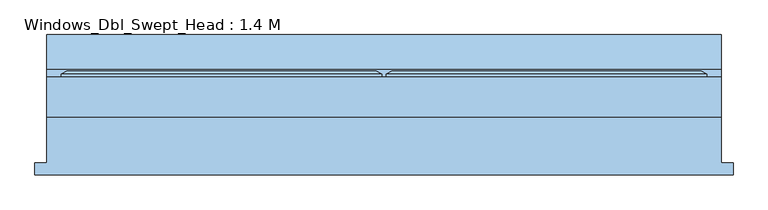
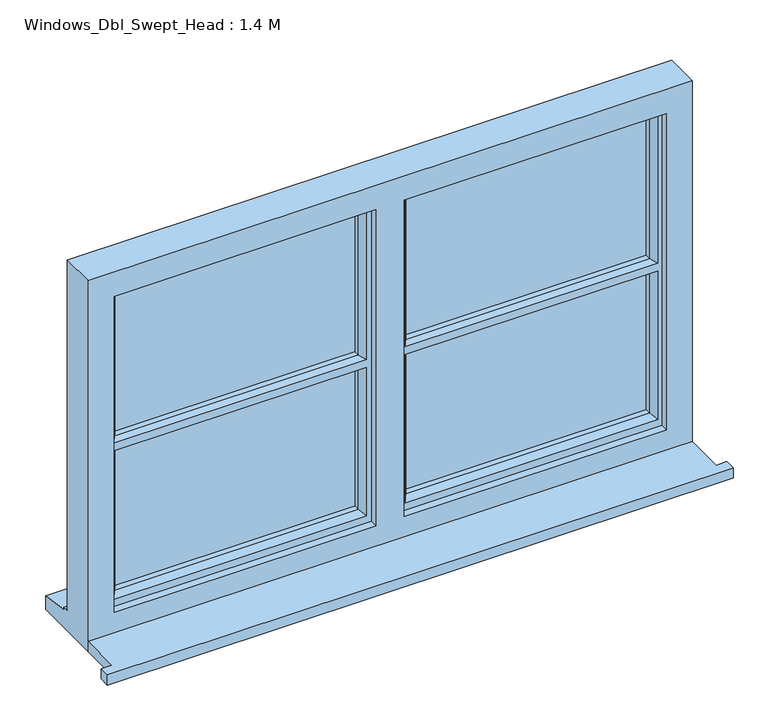
"""IFC4 building model written with IfcOpenShell, lengths in millimetres: window geometry, Windows_Dbl_Swept_Head : 1.4 M."""

from ifc_helpers import new_model, si_unit, frame, origin, place, context, project, spatial, polyline, circle_curve, outline, extrude, faceted_brep, source, transform, mapped, element, save
from ifc_brep_helpers import plane_surface, revolved_surface, advanced_brep


def windows_dbl_swept_head_1_4_m_8667dff2(model_context):
    return source(origin(), model_context, "Body", "SolidModel", [
        extrude(outline(polyline([(-1010.0, -130.8434322), (-1010.0, -105.8434322), (-985.0, -105.8434322), (-985.0, -10.2434322), (415.0, -10.2434322), (415.0, -105.8434322), (440.0, -105.8434322), (440.0, -130.8434322), (-1010.0, -130.8434322)])), frame((0.0, 0.0, 1200.0), z_axis=(0.0, 0.0, 1.0), x_axis=(1.0, 0.0, 0.0)), (0.0, 0.0, 1.0), 25.0),
        extrude(outline(polyline([(345.1480377, 36.7565678), (-240.0, 36.7565678), (-240.0, 60.7565678), (345.1480377, 60.7565678), (345.1480377, 36.7565678)])), frame((0.0, 0.0, 1293.0), z_axis=(0.0, 0.0, 1.0), x_axis=(1.0, 0.0, 0.0)), (0.0, 0.0, 1.0), 365.5),
        extrude(outline(polyline([(345.1480377, 36.7565678), (-240.0, 36.7565678), (-240.0, 60.7565678), (345.1480377, 60.7565678), (345.1480377, 36.7565678)])), frame((0.0, 0.0, 1674.5), z_axis=(0.0, 0.0, 1.0), x_axis=(1.0, 0.0, 0.0)), (0.0, 0.0, 1.0), 365.5),
        extrude(outline(polyline([(-330.0, 36.7565678), (-915.0, 36.7565678), (-915.0, 60.7565678), (-330.0, 60.7565678), (-330.0, 36.7565678)])), frame((0.0, 0.0, 1674.5), z_axis=(0.0, 0.0, 1.0), x_axis=(1.0, 0.0, 0.0)), (0.0, 0.0, 1.0), 365.5),
        extrude(outline(polyline([(-330.0, 36.7565678), (-915.1480377, 36.7565678), (-915.1480377, 60.7565678), (-330.0, 60.7565678), (-330.0, 36.7565678)])), frame((0.0, 0.0, 1292.8519623), z_axis=(0.0, 0.0, 1.0), x_axis=(1.0, 0.0, 0.0)), (0.0, 0.0, 1.0), 365.6480377),
        faceted_brep([(-985.0, -10.2434322, 1200.0), (415.0, -10.2434322, 1200.0), (415.0, -10.2434322, 2110.0), (-985.0, -10.2434322, 2110.0), (-318.0, -10.2434322, 2050.0), (-318.0, -10.2434322, 1275.0), (-925.0, -10.2434322, 1275.0), (-925.0, -10.2434322, 2050.0), (-252.0, -10.2434322, 2050.0), (355.0, -10.2434322, 2050.0), (355.0, -10.2434322, 1275.0), (-252.0, -10.2434322, 1275.0), (-985.0, 72.7565678, 2110.0), (-985.0, 72.7565678, 1251.0), (-985.0, 87.7565678, 1249.68767), (-985.0, 87.7565678, 1244.7449676), (-985.0, 160.2565678, 1233.8088847), (-985.0, 160.2565678, 1200.0), (415.0, 72.7565678, 2110.0), (415.0, 72.7565678, 1251.0), (-945.0, 72.7565678, 2070.0), (-945.0, 72.7565678, 1263.0), (-300.0, 72.7565678, 1263.0), (-300.0, 72.7565678, 2070.0), (-270.0, 72.7565678, 2070.0), (-270.0, 72.7565678, 1263.0), (375.0, 72.7565678, 1263.0), (375.0, 72.7565678, 2070.0), (-945.0, 7.7565678, 2070.0), (-945.0, 7.7565678, 1263.0), (-300.0, 7.7565678, 2070.0), (-300.0, 7.7565678, 1263.0), (-318.0, 7.7565678, 2050.0), (-925.0, 7.7565678, 2050.0), (-925.0, 7.7565678, 1275.0), (-318.0, 7.7565678, 1275.0), (-270.0, 7.7565678, 2070.0), (375.0, 7.7565678, 2070.0), (375.0, 7.7565678, 1263.0), (-270.0, 7.7565678, 1263.0), (355.0, 7.7565678, 2050.0), (-252.0, 7.7565678, 2050.0), (-252.0, 7.7565678, 1275.0), (355.0, 7.7565678, 1275.0), (415.0, 160.2565678, 1200.0), (415.0, 160.2565678, 1233.8088847), (415.0, 87.7565678, 1244.7449676), (415.0, 87.7565678, 1249.68767)], [[[0, 1, 2, 3], [4, 5, 6, 7], [8, 9, 10, 11]], [[0, 3, 12, 13, 14, 15, 16, 17]], [[13, 12, 18, 19], [20, 21, 22, 23], [24, 25, 26, 27]], [[21, 20, 28, 29]], [[28, 30, 31, 29], [32, 33, 34, 35]], [[36, 37, 38, 39], [40, 41, 42, 43]], [[33, 7, 6, 34]], [[12, 3, 2, 18]], [[28, 20, 23, 30]], [[27, 37, 36, 24]], [[7, 33, 32, 4]], [[40, 9, 8, 41]], [[19, 18, 2, 1, 44, 45, 46, 47]], [[27, 26, 38, 37]], [[9, 40, 43, 10]], [[23, 22, 31, 30]], [[25, 24, 36, 39]], [[41, 8, 11, 42]], [[4, 32, 35, 5]], [[44, 1, 0, 17]], [[45, 44, 17, 16]], [[46, 45, 16, 15]], [[47, 46, 15, 14]], [[19, 47, 14, 13]], [[22, 21, 29, 31]], [[26, 25, 39, 38]], [[11, 10, 43, 42]], [[35, 34, 6, 5]]]),
        advanced_brep(
        [(-280.0, 72.7565678, 2080.0), (-280.0, 78.5300705, 2080.0), (-280.0, 78.5300705, 1253.0), (-280.0, 72.7565678, 1253.0), (-270.0, 7.7565678, 2070.0), (-270.0, 72.7565678, 2070.0), (-270.0, 72.7565678, 1263.0), (-270.0, 7.7565678, 1263.0), (-230.0, 22.2494677, 2030.0), (-240.1480377, 7.7565678, 2040.1480377), (-240.1480377, 7.7565678, 1676.3519623), (-230.0, 22.2494677, 1681.5), (-240.1480377, 7.7565678, 1292.8519623), (-230.0, 22.2494677, 1303.0), (-230.0, 22.2494677, 1651.5), (-240.1480377, 7.7565678, 1656.6480377), (-230.0, 36.7565678, 2030.0), (-230.0, 36.7565678, 1681.5), (-230.0, 36.7565678, 1303.0), (-230.0, 36.7565678, 1651.5), (-240.0, 60.7565678, 2040.0), (-240.0, 36.7565678, 2040.0), (-240.0, 36.7565678, 1674.5), (-240.0, 60.7565678, 1674.5), (-240.0, 36.7565678, 1293.0), (-240.0, 60.7565678, 1293.0), (-240.0, 60.7565678, 1658.5), (-240.0, 36.7565678, 1658.5), (-230.0, 60.7565678, 1303.0), (-230.0, 78.5300705, 1303.0), (-230.0, 78.5300705, 1651.5), (-230.0, 60.7565678, 1651.5), (-230.0, 60.7565678, 1681.5), (-230.0, 78.5300705, 1681.5), (-230.0, 78.5300705, 1965.4636992), (-230.0, 60.7565678, 1965.4636992), (-247.4457548, 84.3035732, 2047.4457548), (-230.0, 78.5300705, 2030.0), (-235.0, 80.1847718, 1681.5), (-247.4457548, 84.3035732, 1669.0542452), (-247.4457548, 84.3035732, 1285.5542452), (-247.4457548, 84.3035732, 1663.9457548), (-235.0, 80.1847718, 1651.5), (-269.2153903, 84.3035732, 2069.2153903), (-269.2153903, 84.3035732, 1263.7846097), (385.0, 78.5300705, 1253.0), (385.0, 72.7565678, 1253.0), (375.0, 72.7565678, 1263.0), (375.0, 7.7565678, 1263.0), (345.1480377, 7.7565678, 1292.8519623), (335.0, 22.2494677, 1303.0), (335.0, 36.7565678, 1303.0), (345.0, 36.7565678, 1293.0), (345.0, 60.7565678, 1293.0), (335.0, 60.7565678, 1303.0), (335.0, 78.5300705, 1303.0), (352.4457548, 84.3035732, 1285.5542452), (374.2153903, 84.3035732, 1263.7846097), (385.0, 78.5300705, 2080.0), (385.0, 72.7565678, 2080.0), (375.0, 72.7565678, 2070.0), (375.0, 7.7565678, 2070.0), (345.1480377, 7.7565678, 1656.6480377), (335.0, 22.2494677, 1651.5), (345.1480377, 7.7565678, 2040.1480377), (335.0, 22.2494677, 2030.0), (335.0, 22.2494677, 1681.5), (345.1480377, 7.7565678, 1676.3519623), (335.0, 36.7565678, 1651.5), (335.0, 36.7565678, 2030.0), (335.0, 36.7565678, 1681.5), (345.0, 36.7565678, 1658.5), (345.0, 60.7565678, 1658.5), (345.0, 36.7565678, 2040.0), (345.0, 60.7565678, 2040.0), (345.0, 60.7565678, 1674.5), (345.0, 36.7565678, 1674.5), (335.0, 60.7565678, 1651.5), (335.0, 78.5300705, 1651.5), (335.0, 78.5300705, 1681.5), (335.0, 60.7565678, 1681.5), (335.0, 60.7565678, 1965.4636992), (335.0, 78.5300705, 1965.4636992), (340.0, 80.1847718, 1651.5), (352.4457548, 84.3035732, 1663.9457548), (335.0, 78.5300705, 2030.0), (352.4457548, 84.3035732, 2047.4457548), (352.4457548, 84.3035732, 1669.0542452), (340.0, 80.1847718, 1681.5), (374.2153903, 84.3035732, 2069.2153903)],
        [
            (0, 1),
            (1, 2),
            (2, 3),
            (3, 0),
            (4, 5),
            (5, 6),
            (6, 7),
            (7, 4),
            (8, 9),
            (9, 10),
            (10, 11),
            (11, 8),
            (12, 13),
            (13, 14),
            (14, 15),
            (15, 12),
            (16, 8),
            (11, 17),
            (17, 16),
            (13, 18),
            (18, 19),
            (19, 14),
            (20, 21),
            (21, 22),
            (22, 23),
            (23, 20),
            (24, 25),
            (25, 26),
            (26, 27),
            (27, 24),
            (28, 29),
            (29, 30),
            (30, 31),
            (31, 28),
            (32, 33),
            (33, 34),
            (34, 35),
            (35, 32),
            (36, 37),
            (37, 34),
            (33, 38),
            (38, 39),
            (39, 36),
            (29, 40),
            (40, 41),
            (41, 42),
            (42, 30),
            (1, 43),
            (43, 44),
            (44, 2),
            (2, 45),
            (45, 46),
            (46, 3),
            (6, 47),
            (47, 48),
            (48, 7),
            (12, 49),
            (49, 50),
            (50, 13),
            (50, 51),
            (51, 18),
            (24, 52),
            (52, 53),
            (53, 25),
            (28, 54),
            (54, 55),
            (55, 29),
            (55, 56),
            (56, 40),
            (44, 57),
            (57, 45),
            (45, 58),
            (58, 59),
            (59, 46),
            (47, 60),
            (60, 61),
            (61, 48),
            (49, 62),
            (62, 63),
            (63, 50),
            (64, 65),
            (65, 66),
            (66, 67),
            (67, 64),
            (63, 68),
            (68, 51),
            (65, 69),
            (69, 70),
            (70, 66),
            (52, 71),
            (71, 72),
            (72, 53),
            (73, 74),
            (74, 75),
            (75, 76),
            (76, 73),
            (54, 77),
            (77, 78),
            (78, 55),
            (79, 80),
            (80, 81),
            (81, 82),
            (82, 79),
            (78, 83),
            (83, 84),
            (84, 56),
            (85, 86),
            (86, 87),
            (87, 88),
            (88, 79),
            (82, 85),
            (57, 89),
            (89, 58),
            (0, 59),
            (58, 1),
            (5, 60),
            (4, 61),
            (15, 62),
            (9, 64),
            (67, 10),
            (8, 65),
            (16, 69),
            (27, 71),
            (68, 19),
            (21, 73),
            (76, 22),
            (17, 70),
            (20, 74),
            (72, 26),
            (31, 77),
            (23, 75),
            (80, 32),
            (35, 81, circle_curve(frame((52.5, 60.7565678, 1325.0), z_axis=(0.0, 1.0, 0.0), x_axis=(1.0, 0.0, 0.0)), 700.0)),
            (36, 86),
            (85, 37),
            (43, 89),
            (84, 41),
            (39, 87),
            (38, 88),
            (11, 66),
            (14, 63),
            (42, 83),
            (82, 34, circle_curve(frame((52.5, 78.5300705, 1325.0), z_axis=(0.0, -1.0, 0.0), x_axis=(1.0, 0.0, 0.0)), 700.0)),
        ],
        [
            plane_surface(frame((-280.0, 78.5300705, 2080.0), z_axis=(-1.0, 0.0, 0.0), x_axis=(0.0, 0.0, -1.0))),
            plane_surface(frame((-270.0, 72.7565678, 2070.0), z_axis=(-1.0, 0.0, 0.0), x_axis=(0.0, 0.0, -1.0))),
            plane_surface(frame((-240.1480377, 7.7565678, 2040.1480377), z_axis=(0.8191520442889492, -0.5735764363511071, 0.0), x_axis=(0.0, 0.0, -1.0))),
            plane_surface(frame((-230.0, 22.2494677, 2030.0), z_axis=(1.0, 0.0, 0.0), x_axis=(0.0, 0.0, -1.0))),
            plane_surface(frame((-240.0, 36.7565678, 2040.0), z_axis=(1.0, 0.0, 0.0), x_axis=(0.0, 0.0, -1.0))),
            plane_surface(frame((-230.0, 60.7565678, 2030.0), z_axis=(1.0, 0.0, 0.0), x_axis=(0.0, 0.0, -1.0))),
            plane_surface(frame((-230.0, 78.5300705, 2030.0), z_axis=(0.31418232948755237, 0.9493626619147053, 0.0), x_axis=(0.0, 0.0, -1.0))),
            plane_surface(frame((-269.2153903, 84.3035732, 2069.2153903), z_axis=(-0.47196942945730275, 0.8816149146071363, 0.0), x_axis=(0.0, 0.0, -1.0))),
            plane_surface(frame((-280.0, 78.5300705, 1253.0), z_axis=(0.0, 0.0, -1.0), x_axis=(1.0, 0.0, 0.0))),
            plane_surface(frame((-270.0, 72.7565678, 1263.0), z_axis=(0.0, 0.0, -1.0), x_axis=(1.0, 0.0, 0.0))),
            plane_surface(frame((-240.1480377, 7.7565678, 1292.8519623), z_axis=(0.0, -0.5735764363511044, 0.819152044288951), x_axis=(1.0, 0.0, 0.0))),
            plane_surface(frame((-230.0, 22.2494677, 1303.0), z_axis=(0.0, 0.0, 1.0), x_axis=(1.0, 0.0, 0.0))),
            plane_surface(frame((-240.0, 36.7565678, 1293.0), z_axis=(0.0, 0.0, 1.0), x_axis=(1.0, 0.0, 0.0))),
            plane_surface(frame((-230.0, 60.7565678, 1303.0), z_axis=(0.0, 0.0, 1.0), x_axis=(1.0, 0.0, 0.0))),
            plane_surface(frame((-230.0, 78.5300705, 1303.0), z_axis=(0.0, 0.9493626619147063, 0.31418232948754926), x_axis=(1.0, 0.0, 0.0))),
            plane_surface(frame((-269.2153903, 84.3035732, 1263.7846097), z_axis=(0.0, 0.8816149146071347, -0.47196942945730563), x_axis=(1.0, 0.0, 0.0))),
            plane_surface(frame((385.0, 78.5300705, 1253.0), z_axis=(1.0, 0.0, 0.0), x_axis=(0.0, 0.0, 1.0))),
            plane_surface(frame((375.0, 72.7565678, 1263.0), z_axis=(1.0, 0.0, 0.0), x_axis=(0.0, 0.0, 1.0))),
            plane_surface(frame((345.1480377, 7.7565678, 1292.8519623), z_axis=(-0.8191520442889529, -0.5735764363511018, 0.0), x_axis=(0.0, 0.0, 1.0))),
            plane_surface(frame((335.0, 22.2494677, 1303.0), z_axis=(-1.0, 0.0, 0.0), x_axis=(0.0, 0.0, 1.0))),
            plane_surface(frame((345.0, 36.7565678, 1293.0), z_axis=(-1.0, 0.0, 0.0), x_axis=(0.0, 0.0, 1.0))),
            plane_surface(frame((335.0, 60.7565678, 1303.0), z_axis=(-1.0, 0.0, 0.0), x_axis=(0.0, 0.0, 1.0))),
            plane_surface(frame((335.0, 78.5300705, 1303.0), z_axis=(-0.3141823294875462, 0.9493626619147074, 0.0), x_axis=(0.0, 0.0, 1.0))),
            plane_surface(frame((374.2153903, 84.3035732, 1263.7846097), z_axis=(0.4719694294573085, 0.8816149146071331, 0.0), x_axis=(0.0, 0.0, 1.0))),
            plane_surface(frame((385.0, 78.5300705, 2080.0), z_axis=(0.0, 0.0, 1.0), x_axis=(-1.0, 0.0, 0.0))),
            plane_surface(frame((385.0, 72.7565678, 2080.0), z_axis=(0.0, -1.0, 0.0), x_axis=(-1.0, 0.0, 0.0))),
            plane_surface(frame((375.0, 72.7565678, 2070.0), z_axis=(0.0, 0.0, 1.0), x_axis=(-1.0, 0.0, 0.0))),
            plane_surface(frame((375.0, 7.7565678, 2070.0), z_axis=(0.0, -1.0, 0.0), x_axis=(-1.0, 0.0, 0.0))),
            plane_surface(frame((345.1480377, 7.7565678, 2040.1480377), z_axis=(0.0, -0.5735764363511044, -0.819152044288951), x_axis=(-1.0, 0.0, 0.0))),
            plane_surface(frame((335.0, 22.2494677, 2030.0), z_axis=(0.0, 0.0, -1.0), x_axis=(-1.0, 0.0, 0.0))),
            plane_surface(frame((335.0, 36.7565678, 2030.0), z_axis=(0.0, 1.0, 0.0), x_axis=(-1.0, 0.0, 0.0))),
            plane_surface(frame((345.0, 36.7565678, 2040.0), z_axis=(0.0, 0.0, -1.0), x_axis=(-1.0, 0.0, 0.0))),
            plane_surface(frame((345.0, 60.7565678, 2040.0), z_axis=(0.0, -1.0, 0.0), x_axis=(-1.0, 0.0, 0.0))),
            plane_surface(frame((335.0, 78.5300705, 2030.0), z_axis=(0.0, 0.9493626619147064, -0.3141823294875493), x_axis=(-1.0, 0.0, 0.0))),
            plane_surface(frame((352.4457548, 84.3035732, 2047.4457548), z_axis=(0.0, 1.0, 0.0), x_axis=(-1.0, 0.0, 0.0))),
            plane_surface(frame((374.2153903, 84.3035732, 2069.2153903), z_axis=(0.0, 0.8816149146071347, 0.47196942945730563), x_axis=(-1.0, 0.0, 0.0))),
            plane_surface(frame((352.4457548, 84.3035732, 1669.0542452), z_axis=(0.0, 0.9493626619145938, 0.3141823294878896), x_axis=(-1.0, 0.0, 0.0))),
            plane_surface(frame((352.4457548, 80.1847718, 1681.5), z_axis=(0.0, 0.0, 1.0), x_axis=(-1.0, 0.0, 0.0))),
            plane_surface(frame((352.4457548, 60.7565678, 1674.5), z_axis=(0.0, 0.0, 1.0), x_axis=(-1.0, 0.0, 0.0))),
            plane_surface(frame((352.4457548, 36.7565678, 1681.5), z_axis=(0.0, 0.0, 1.0), x_axis=(-1.0, 0.0, 0.0))),
            plane_surface(frame((352.4457548, 22.2494677, 1681.5), z_axis=(0.0, -0.33472142672711697, 0.9423171262848634), x_axis=(-1.0, 0.0, 0.0))),
            plane_surface(frame((352.4457548, 7.7565678, 1656.6480377), z_axis=(0.0, -0.33472142672499106, -0.9423171262856186), x_axis=(-1.0, 0.0, 0.0))),
            plane_surface(frame((352.4457548, 22.2494677, 1651.5), z_axis=(0.0, 0.0, -1.0), x_axis=(-1.0, 0.0, 0.0))),
            plane_surface(frame((352.4457548, 36.7565678, 1658.5), z_axis=(0.0, 0.0, -1.0), x_axis=(-1.0, 0.0, 0.0))),
            plane_surface(frame((352.4457548, 60.7565678, 1651.5), z_axis=(0.0, 0.0, -1.0), x_axis=(-1.0, 0.0, 0.0))),
            plane_surface(frame((352.4457548, 80.1847718, 1651.5), z_axis=(0.0, 0.9493626619148547, -0.31418232948710106), x_axis=(-1.0, 0.0, 0.0))),
            plane_surface(frame((-230.0, 78.5300705, 2030.0), z_axis=(0.0, 1.0, 0.0), x_axis=(0.0, 0.0, 1.0))),
            revolved_surface(polyline([(752.5, 78.5300705, 1325.0), (752.5, 60.7565678, 1325.0)]), (52.5, 78.5300705, 1325.0), (0.0, 1.0, 0.0)),
        ],
        [
            (0, [[1, 2, 3, 4]]),
            (1, [[5, 6, 7, 8]]),
            (2, [[9, 10, 11, 12]]),
            (2, [[13, 14, 15, 16]]),
            (3, [[17, -12, 18, 19]]),
            (3, [[20, 21, 22, -14]]),
            (4, [[23, 24, 25, 26]]),
            (4, [[27, 28, 29, 30]]),
            (5, [[31, 32, 33, 34]]),
            (5, [[35, 36, 37, 38]]),
            (6, [[39, 40, -36, 41, 42, 43]]),
            (6, [[44, 45, 46, 47, -32]]),
            (7, [[-2, 48, 49, 50]]),
            (8, [[-3, 51, 52, 53]]),
            (9, [[-7, 54, 55, 56]]),
            (10, [[-13, 57, 58, 59]]),
            (11, [[-20, -59, 60, 61]]),
            (12, [[-27, 62, 63, 64]]),
            (13, [[-31, 65, 66, 67]]),
            (14, [[-44, -67, 68, 69]]),
            (15, [[-50, 70, 71, -51]]),
            (16, [[-52, 72, 73, 74]]),
            (17, [[-55, 75, 76, 77]]),
            (18, [[-58, 78, 79, 80]]),
            (18, [[81, 82, 83, 84]]),
            (19, [[-60, -80, 85, 86]]),
            (19, [[87, 88, 89, -82]]),
            (20, [[-63, 90, 91, 92]]),
            (20, [[93, 94, 95, 96]]),
            (21, [[-66, 97, 98, 99]]),
            (21, [[100, 101, 102, 103]]),
            (22, [[-68, -99, 104, 105, 106]]),
            (22, [[107, 108, 109, 110, -103, 111]]),
            (23, [[-71, 112, 113, -72]]),
            (24, [[-1, 114, -73, 115]]),
            (25, [[-4, -53, -74, -114], [-6, 116, -75, -54]]),
            (26, [[-5, 117, -76, -116]]),
            (27, [[-8, -56, -77, -117], [-57, -16, 118, -78], [119, -84, 120, -10]]),
            (28, [[-9, 121, -81, -119]]),
            (29, [[-17, 122, -87, -121]]),
            (30, [[-62, -30, 123, -90], [-61, -86, 124, -21]]),
            (30, [[125, -96, 126, -24], [-122, -19, 127, -88]]),
            (31, [[-23, 128, -93, -125]]),
            (32, [[-64, -92, 129, -28], [-65, -34, 130, -97]]),
            (32, [[-128, -26, 131, -94], [132, -38, 133, -101]]),
            (33, [[-39, 134, -107, 135]]),
            (34, [[-49, 136, -112, -70], [-69, -106, 137, -45], [-134, -43, 138, -108]]),
            (35, [[-48, -115, -113, -136]]),
            (36, [[-138, -42, 139, -109]]),
            (37, [[-132, -100, -110, -139, -41, -35]]),
            (38, [[-25, -126, -95, -131]]),
            (39, [[140, -89, -127, -18]]),
            (40, [[-120, -83, -140, -11]]),
            (41, [[-118, -15, 141, -79]]),
            (42, [[-141, -22, -124, -85]]),
            (43, [[-29, -129, -91, -123]]),
            (44, [[-130, -33, -47, 142, -104, -98]]),
            (45, [[-137, -105, -142, -46]]),
            (46, [[143, -40, -135, -111]]),
            (47, [[-133, -37, -143, -102]]),
        ],
    ),
        advanced_brep(
        [(-330.0, 60.7565678, 2040.0), (-915.0, 60.7565678, 2040.0), (-915.0, 60.7565678, 1674.5), (-330.0, 60.7565678, 1674.5), (-905.0, 60.7565678, 1965.4636992), (-340.0, 60.7565678, 1965.4636992), (-340.0, 60.7565678, 1681.5), (-905.0, 60.7565678, 1681.5), (-915.0, 60.7565678, 1293.0), (-330.0, 60.7565678, 1293.0), (-330.0, 60.7565678, 1658.5), (-915.0, 60.7565678, 1658.5), (-340.0, 60.7565678, 1303.0), (-905.0, 60.7565678, 1303.0), (-905.0, 60.7565678, 1651.5), (-340.0, 60.7565678, 1651.5), (-955.0, 72.7565678, 2080.0), (-955.0, 78.5300705, 2080.0), (-955.0, 78.5300705, 1253.0), (-955.0, 72.7565678, 1253.0), (-945.0, 7.7565678, 2070.0), (-945.0, 72.7565678, 2070.0), (-945.0, 72.7565678, 1263.0), (-945.0, 7.7565678, 1263.0), (-905.0, 22.2494677, 2030.0), (-915.1480377, 7.7565678, 2040.1480377), (-915.1480377, 7.7565678, 1676.3519623), (-905.0, 22.2494677, 1681.5), (-915.1480377, 7.7565678, 1292.8519623), (-905.0, 22.2494677, 1303.0), (-905.0, 22.2494677, 1651.5), (-915.1480377, 7.7565678, 1656.6480377), (-905.0, 36.7565678, 2030.0), (-905.0, 36.7565678, 1681.5), (-905.0, 36.7565678, 1303.0), (-905.0, 36.7565678, 1651.5), (-915.0, 36.7565678, 2040.0), (-915.0, 36.7565678, 1674.5), (-915.0, 36.7565678, 1293.0), (-915.0, 36.7565678, 1658.5), (-905.0, 78.5300705, 1303.0), (-905.0, 78.5300705, 1651.5), (-905.0, 78.5300705, 1681.5), (-905.0, 78.5300705, 1965.4636992), (-922.4457548, 84.3035732, 2047.4457548), (-905.0, 78.5300705, 2030.0), (-910.0, 80.1847718, 1681.5), (-922.4457548, 84.3035732, 1669.0542452), (-922.4457548, 84.3035732, 1285.5542452), (-922.4457548, 84.3035732, 1663.9457548), (-910.0, 80.1847718, 1651.5), (-944.2153903, 84.3035732, 2069.2153903), (-944.2153903, 84.3035732, 1263.7846097), (-290.0, 78.5300705, 1253.0), (-290.0, 72.7565678, 1253.0), (-300.0, 72.7565678, 1263.0), (-300.0, 7.7565678, 1263.0), (-329.8519623, 7.7565678, 1292.8519623), (-340.0, 22.2494677, 1303.0), (-340.0, 36.7565678, 1303.0), (-330.0, 36.7565678, 1293.0), (-340.0, 78.5300705, 1303.0), (-322.5542452, 84.3035732, 1285.5542452), (-300.7846097, 84.3035732, 1263.7846097), (-290.0, 78.5300705, 2080.0), (-290.0, 72.7565678, 2080.0), (-300.0, 72.7565678, 2070.0), (-300.0, 7.7565678, 2070.0), (-329.8519623, 7.7565678, 1656.6480377), (-340.0, 22.2494677, 1651.5), (-329.8519623, 7.7565678, 2040.1480377), (-340.0, 22.2494677, 2030.0), (-340.0, 22.2494677, 1681.5), (-329.8519623, 7.7565678, 1676.3519623), (-340.0, 36.7565678, 1651.5), (-340.0, 36.7565678, 2030.0), (-340.0, 36.7565678, 1681.5), (-330.0, 36.7565678, 1658.5), (-330.0, 36.7565678, 2040.0), (-330.0, 36.7565678, 1674.5), (-340.0, 78.5300705, 1651.5), (-340.0, 78.5300705, 1681.5), (-340.0, 78.5300705, 1965.4636992), (-335.0, 80.1847718, 1651.5), (-322.5542452, 84.3035732, 1663.9457548), (-340.0, 78.5300705, 2030.0), (-322.5542452, 84.3035732, 2047.4457548), (-322.5542452, 84.3035732, 1669.0542452), (-335.0, 80.1847718, 1681.5), (-300.7846097, 84.3035732, 2069.2153903)],
        [
            (0, 1),
            (1, 2),
            (2, 3),
            (3, 0),
            (4, 5, circle_curve(frame((-622.5, 60.7565678, 1325.0), z_axis=(0.0, 1.0, 0.0), x_axis=(1.0, 0.0, 0.0)), 700.0)),
            (5, 6),
            (6, 7),
            (7, 4),
            (8, 9),
            (9, 10),
            (10, 11),
            (11, 8),
            (12, 13),
            (13, 14),
            (14, 15),
            (15, 12),
            (16, 17),
            (17, 18),
            (18, 19),
            (19, 16),
            (20, 21),
            (21, 22),
            (22, 23),
            (23, 20),
            (24, 25),
            (25, 26),
            (26, 27),
            (27, 24),
            (28, 29),
            (29, 30),
            (30, 31),
            (31, 28),
            (32, 24),
            (27, 33),
            (33, 32),
            (29, 34),
            (34, 35),
            (35, 30),
            (1, 36),
            (36, 37),
            (37, 2),
            (38, 8),
            (11, 39),
            (39, 38),
            (13, 40),
            (40, 41),
            (41, 14),
            (7, 42),
            (42, 43),
            (43, 4),
            (44, 45),
            (45, 43),
            (42, 46),
            (46, 47),
            (47, 44),
            (40, 48),
            (48, 49),
            (49, 50),
            (50, 41),
            (17, 51),
            (51, 52),
            (52, 18),
            (18, 53),
            (53, 54),
            (54, 19),
            (22, 55),
            (55, 56),
            (56, 23),
            (28, 57),
            (57, 58),
            (58, 29),
            (58, 59),
            (59, 34),
            (38, 60),
            (60, 9),
            (12, 61),
            (61, 40),
            (61, 62),
            (62, 48),
            (52, 63),
            (63, 53),
            (53, 64),
            (64, 65),
            (65, 54),
            (55, 66),
            (66, 67),
            (67, 56),
            (57, 68),
            (68, 69),
            (69, 58),
            (70, 71),
            (71, 72),
            (72, 73),
            (73, 70),
            (69, 74),
            (74, 59),
            (71, 75),
            (75, 76),
            (76, 72),
            (60, 77),
            (77, 10),
            (78, 0),
            (3, 79),
            (79, 78),
            (15, 80),
            (80, 61),
            (81, 6),
            (5, 82),
            (82, 81),
            (80, 83),
            (83, 84),
            (84, 62),
            (85, 86),
            (86, 87),
            (87, 88),
            (88, 81),
            (82, 85),
            (63, 89),
            (89, 64),
            (16, 65),
            (64, 17),
            (21, 66),
            (20, 67),
            (31, 68),
            (25, 70),
            (73, 26),
            (24, 71),
            (32, 75),
            (39, 77),
            (74, 35),
            (36, 78),
            (79, 37),
            (33, 76),
            (44, 86),
            (85, 45),
            (51, 89),
            (84, 49),
            (47, 87),
            (46, 88),
            (83, 50),
            (69, 30),
            (72, 27),
            (82, 43, circle_curve(frame((-622.5, 78.5300705, 1325.0), z_axis=(0.0, -1.0, 0.0), x_axis=(1.0, 0.0, 0.0)), 700.0)),
        ],
        [
            plane_surface(frame((345.0, 60.7565678, 2040.0), z_axis=(0.0, -1.0, 0.0), x_axis=(-1.0, 0.0, 0.0))),
            plane_surface(frame((-955.0, 78.5300705, 2080.0), z_axis=(-1.0, 0.0, 0.0), x_axis=(0.0, 0.0, -1.0))),
            plane_surface(frame((-945.0, 72.7565678, 2070.0), z_axis=(-1.0, 0.0, 0.0), x_axis=(0.0, 0.0, -1.0))),
            plane_surface(frame((-915.1480377, 7.7565678, 2040.1480377), z_axis=(0.8191520442889492, -0.5735764363511071, 0.0), x_axis=(0.0, 0.0, -1.0))),
            plane_surface(frame((-905.0, 22.2494677, 2030.0), z_axis=(1.0, 0.0, 0.0), x_axis=(0.0, 0.0, -1.0))),
            plane_surface(frame((-915.0, 36.7565678, 2040.0), z_axis=(1.0, 0.0, 0.0), x_axis=(0.0, 0.0, -1.0))),
            plane_surface(frame((-905.0, 60.7565678, 2030.0), z_axis=(1.0, 0.0, 0.0), x_axis=(0.0, 0.0, -1.0))),
            plane_surface(frame((-905.0, 78.5300705, 2030.0), z_axis=(0.31418232948755237, 0.9493626619147053, 0.0), x_axis=(0.0, 0.0, -1.0))),
            plane_surface(frame((-944.2153903, 84.3035732, 2069.2153903), z_axis=(-0.47196942945730275, 0.8816149146071363, 0.0), x_axis=(0.0, 0.0, -1.0))),
            plane_surface(frame((-955.0, 78.5300705, 1253.0), z_axis=(0.0, 0.0, -1.0), x_axis=(1.0, 0.0, 0.0))),
            plane_surface(frame((-945.0, 72.7565678, 1263.0), z_axis=(0.0, 0.0, -1.0), x_axis=(1.0, 0.0, 0.0))),
            plane_surface(frame((-915.1480377, 7.7565678, 1292.8519623), z_axis=(0.0, -0.5735764363511044, 0.819152044288951), x_axis=(1.0, 0.0, 0.0))),
            plane_surface(frame((-905.0, 22.2494677, 1303.0), z_axis=(0.0, 0.0, 1.0), x_axis=(1.0, 0.0, 0.0))),
            plane_surface(frame((-915.0, 36.7565678, 1293.0), z_axis=(0.0, 0.0, 1.0), x_axis=(1.0, 0.0, 0.0))),
            plane_surface(frame((-905.0, 60.7565678, 1303.0), z_axis=(0.0, 0.0, 1.0), x_axis=(1.0, 0.0, 0.0))),
            plane_surface(frame((-905.0, 78.5300705, 1303.0), z_axis=(0.0, 0.9493626619147063, 0.31418232948754926), x_axis=(1.0, 0.0, 0.0))),
            plane_surface(frame((-944.2153903, 84.3035732, 1263.7846097), z_axis=(0.0, 0.8816149146071347, -0.47196942945730563), x_axis=(1.0, 0.0, 0.0))),
            plane_surface(frame((-290.0, 78.5300705, 1253.0), z_axis=(1.0, 0.0, 0.0), x_axis=(0.0, 0.0, 1.0))),
            plane_surface(frame((-300.0, 72.7565678, 1263.0), z_axis=(1.0, 0.0, 0.0), x_axis=(0.0, 0.0, 1.0))),
            plane_surface(frame((-329.8519623, 7.7565678, 1292.8519623), z_axis=(-0.8191520442889529, -0.5735764363511018, 0.0), x_axis=(0.0, 0.0, 1.0))),
            plane_surface(frame((-340.0, 22.2494677, 1303.0), z_axis=(-1.0, 0.0, 0.0), x_axis=(0.0, 0.0, 1.0))),
            plane_surface(frame((-330.0, 36.7565678, 1293.0), z_axis=(-1.0, 0.0, 0.0), x_axis=(0.0, 0.0, 1.0))),
            plane_surface(frame((-340.0, 60.7565678, 1303.0), z_axis=(-1.0, 0.0, 0.0), x_axis=(0.0, 0.0, 1.0))),
            plane_surface(frame((-340.0, 78.5300705, 1303.0), z_axis=(-0.3141823294875462, 0.9493626619147074, 0.0), x_axis=(0.0, 0.0, 1.0))),
            plane_surface(frame((-300.7846097, 84.3035732, 1263.7846097), z_axis=(0.4719694294573085, 0.8816149146071331, 0.0), x_axis=(0.0, 0.0, 1.0))),
            plane_surface(frame((-290.0, 78.5300705, 2080.0), z_axis=(0.0, 0.0, 1.0), x_axis=(-1.0, 0.0, 0.0))),
            plane_surface(frame((-290.0, 72.7565678, 2080.0), z_axis=(0.0, -1.0, 0.0), x_axis=(-1.0, 0.0, 0.0))),
            plane_surface(frame((-300.0, 72.7565678, 2070.0), z_axis=(0.0, 0.0, 1.0), x_axis=(-1.0, 0.0, 0.0))),
            plane_surface(frame((-300.0, 7.7565678, 2070.0), z_axis=(0.0, -1.0, 0.0), x_axis=(-1.0, 0.0, 0.0))),
            plane_surface(frame((-329.8519623, 7.7565678, 2040.1480377), z_axis=(0.0, -0.5735764363511044, -0.819152044288951), x_axis=(-1.0, 0.0, 0.0))),
            plane_surface(frame((-340.0, 22.2494677, 2030.0), z_axis=(0.0, 0.0, -1.0), x_axis=(-1.0, 0.0, 0.0))),
            plane_surface(frame((-340.0, 36.7565678, 2030.0), z_axis=(0.0, 1.0, 0.0), x_axis=(-1.0, 0.0, 0.0))),
            plane_surface(frame((-330.0, 36.7565678, 2040.0), z_axis=(0.0, 0.0, -1.0), x_axis=(-1.0, 0.0, 0.0))),
            plane_surface(frame((-340.0, 78.5300705, 2030.0), z_axis=(0.0, 0.9493626619147064, -0.3141823294875493), x_axis=(-1.0, 0.0, 0.0))),
            plane_surface(frame((-322.5542452, 84.3035732, 2047.4457548), z_axis=(0.0, 1.0, 0.0), x_axis=(-1.0, 0.0, 0.0))),
            plane_surface(frame((-300.7846097, 84.3035732, 2069.2153903), z_axis=(0.0, 0.8816149146071347, 0.47196942945730563), x_axis=(-1.0, 0.0, 0.0))),
            plane_surface(frame((-922.4457548, 80.1847718, 1681.5), z_axis=(0.0, 0.9493626619144715, 0.31418232948825914), x_axis=(1.0, 0.0, 0.0))),
            plane_surface(frame((-922.4457548, 84.3035732, 1663.9457548), z_axis=(0.0, 0.949362661914977, -0.3141823294867314), x_axis=(1.0, 0.0, 0.0))),
            plane_surface(frame((-922.4457548, 80.1847718, 1651.5), z_axis=(0.0, 0.0, -1.0), x_axis=(1.0, 0.0, 0.0))),
            plane_surface(frame((-922.4457548, 60.7565678, 1658.5), z_axis=(0.0, 0.0, -1.0), x_axis=(1.0, 0.0, 0.0))),
            plane_surface(frame((-922.4457548, 36.7565678, 1651.5), z_axis=(0.0, 0.0, -1.0), x_axis=(1.0, 0.0, 0.0))),
            plane_surface(frame((-922.4457548, 22.2494677, 1651.5), z_axis=(0.0, -0.3347214267259168, -0.9423171262852897), x_axis=(1.0, 0.0, 0.0))),
            plane_surface(frame((-922.4457548, 7.7565678, 1676.3519623), z_axis=(0.0, -0.33472142672616695, 0.9423171262852009), x_axis=(1.0, 0.0, 0.0))),
            plane_surface(frame((-922.4457548, 22.2494677, 1681.5), z_axis=(0.0, 0.0, 1.0), x_axis=(1.0, 0.0, 0.0))),
            plane_surface(frame((-922.4457548, 36.7565678, 1674.5), z_axis=(0.0, 0.0, 1.0), x_axis=(1.0, 0.0, 0.0))),
            plane_surface(frame((-922.4457548, 60.7565678, 1681.5), z_axis=(0.0, 0.0, 1.0), x_axis=(1.0, 0.0, 0.0))),
            plane_surface(frame((-230.0, 78.5300705, 2030.0), z_axis=(0.0, 1.0, 0.0), x_axis=(0.0, 0.0, 1.0))),
            revolved_surface(polyline([(77.5, 78.5300705, 1325.0), (77.5, 60.7565678, 1325.0)]), (-622.5, 72.7565678, 1325.0), (0.0, 1.0, 0.0)),
        ],
        [
            (0, [[1, 2, 3, 4], [5, 6, 7, 8]]),
            (0, [[9, 10, 11, 12], [13, 14, 15, 16]]),
            (1, [[17, 18, 19, 20]]),
            (2, [[21, 22, 23, 24]]),
            (3, [[25, 26, 27, 28]]),
            (3, [[29, 30, 31, 32]]),
            (4, [[33, -28, 34, 35]]),
            (4, [[36, 37, 38, -30]]),
            (5, [[39, 40, 41, -2]]),
            (5, [[42, -12, 43, 44]]),
            (6, [[45, 46, 47, -14]]),
            (6, [[48, 49, 50, -8]]),
            (7, [[51, 52, -49, 53, 54, 55]]),
            (7, [[56, 57, 58, 59, -46]]),
            (8, [[-18, 60, 61, 62]]),
            (9, [[-19, 63, 64, 65]]),
            (10, [[-23, 66, 67, 68]]),
            (11, [[-29, 69, 70, 71]]),
            (12, [[-36, -71, 72, 73]]),
            (13, [[-42, 74, 75, -9]]),
            (14, [[-45, -13, 76, 77]]),
            (15, [[-56, -77, 78, 79]]),
            (16, [[-62, 80, 81, -63]]),
            (17, [[-64, 82, 83, 84]]),
            (18, [[-67, 85, 86, 87]]),
            (19, [[-70, 88, 89, 90]]),
            (19, [[91, 92, 93, 94]]),
            (20, [[-72, -90, 95, 96]]),
            (20, [[97, 98, 99, -92]]),
            (21, [[-75, 100, 101, -10]]),
            (21, [[102, -4, 103, 104]]),
            (22, [[-76, -16, 105, 106]]),
            (22, [[107, -6, 108, 109]]),
            (23, [[-78, -106, 110, 111, 112]]),
            (23, [[113, 114, 115, 116, -109, 117]]),
            (24, [[-81, 118, 119, -82]]),
            (25, [[-17, 120, -83, 121]]),
            (26, [[-20, -65, -84, -120], [-22, 122, -85, -66]]),
            (27, [[-21, 123, -86, -122]]),
            (28, [[-24, -68, -87, -123], [-69, -32, 124, -88], [125, -94, 126, -26]]),
            (29, [[-25, 127, -91, -125]]),
            (30, [[-33, 128, -97, -127]]),
            (31, [[-74, -44, 129, -100], [-73, -96, 130, -37]]),
            (31, [[131, -104, 132, -40], [-128, -35, 133, -98]]),
            (32, [[-39, -1, -102, -131]]),
            (33, [[-51, 134, -113, 135]]),
            (34, [[-61, 136, -118, -80], [-79, -112, 137, -57], [-134, -55, 138, -114]]),
            (35, [[-60, -121, -119, -136]]),
            (36, [[-138, -54, 139, -115]]),
            (37, [[-137, -111, 140, -58]]),
            (38, [[-15, -47, -59, -140, -110, -105]]),
            (39, [[-43, -11, -101, -129]]),
            (40, [[141, -38, -130, -95]]),
            (41, [[-124, -31, -141, -89]]),
            (42, [[-126, -93, 142, -27]]),
            (43, [[-142, -99, -133, -34]]),
            (44, [[-41, -132, -103, -3]]),
            (45, [[-7, -107, -116, -139, -53, -48]]),
            (46, [[143, -52, -135, -117]]),
            (47, [[-5, -50, -143, -108]]),
        ],
    ),
    ])


if __name__ == "__main__":
    model = new_model("IFC4")
    model_context = context("Model", 3, world=origin())
    ifc_project = project(units=[si_unit("LENGTHUNIT", "METRE", prefix="MILLI")], contexts=[model_context])
    site = spatial("IfcSite", under=ifc_project)
    building = spatial("IfcBuilding", under=site)
    placement = place(None, origin())
    windows_dbl_swept_head_1_4_m_shape = windows_dbl_swept_head_1_4_m_8667dff2(model_context)
    element("IfcWindow", 1, ObjectType="Windows_Dbl_Swept_Head : 1.4 M", at=placement, inside=building, context=model_context, shape_type="MappedRepresentation", body=[
        mapped(windows_dbl_swept_head_1_4_m_shape, transform((0.0, 0.0, 0.0), x_axis=(1.0, 0.0, 0.0), y_axis=(0.0, 1.0, 0.0), z_axis=(0.0, 0.0, 1.0))),
    ])
    save(model, "model.ifc")

# Revit data of these elements
# Type "Windows_Dbl_Swept_Head : 1.4 M"
#   Type Mark = "66"
#   Operation = "DoublePanelVertical"
#   Construction Type Id = "GSP4R"
#   Manufacturer = "Revit"
#   Keynote = "L10"
#   Analytic Construction = "1/8 in Pilkington single glazing"
#   Wrap Layers (Ext) from Ext = 0.1025 m
#   Wrap Layers (Int) from Ext = 0.1775 m
#   Window Board Projection = 0.025 m
#   Window Board Extension = 0.025 m
#   Visual Light Transmittance = 0.9
#   Solar Heat Gain Coefficient = 0.78
#   Rough Width = 1.4 m
#   Rough Height = 0.91 m
#   Radius - Swept Head = 0.7 m
#   Height = 0.91 m
#   Width = 1.4 m
#   Heat Transfer Coefficient (U) = 3.6886 W/(m²·K)
#   Glazing Thickness = 0.024 m
#   FrameOffset - External = 0.05 m
#   Frame Depth = 0.065 m
#   Default Head Height = 2.11 m
#   Cill Depth = 0.0875 m
#   Cavity Closer Width = 0.05 m
#   Cavity Closer Offset from Ext = 0.1025 m
#   Cavity Closer Depth = 0.085 m
#   Vis - Cavity Closers = yes
#   Define Thermal Properties by = 1
#   Material Trim = Window Frame
#   Material Glass = Glass
#   Material Frame = Window Frame
#   Wall Closure = (empty or 0)
# Element 1 (IfcWindow, "Windows_Dbl_Swept_Head : 1.4 M")
#   Materials on its faces: "Window Frame", "Glass"
# Materials
#   "Window Frame": colour RGB 249 249 249, transparency 0, Keynote = "L10", Cost = 0
#   "Glass": class "Glass", colour RGB 0 128 192, transparency 0.9, Description = "Soda Lime Glass", Cost = 0
